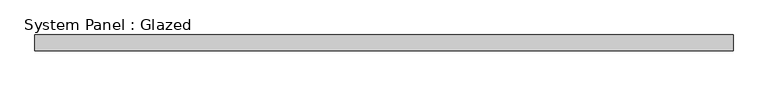
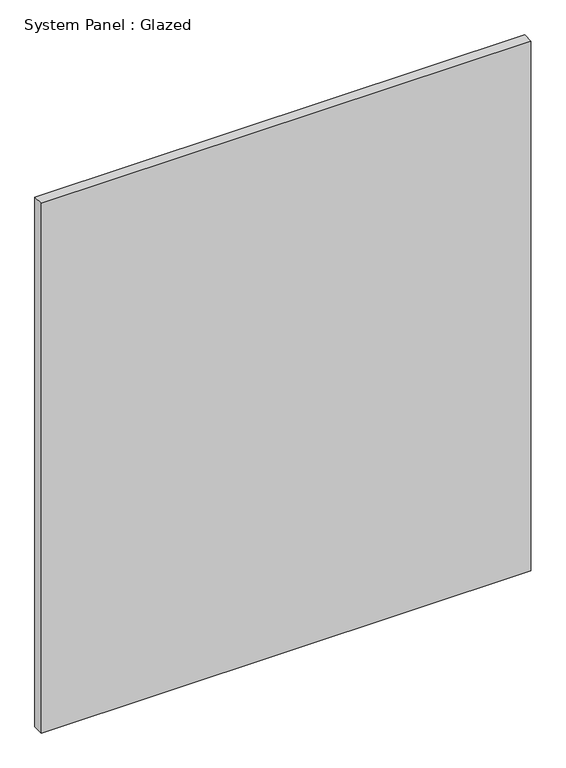
"""IFC4 building model written with IfcOpenShell, lengths in millimetres: plate geometry, System Panel : Glazed."""

from ifc_helpers import new_model, si_unit, origin, origin_with_axes, place, context, project, spatial, polyline, outline, extrude, source, transform, mapped, element, save


def system_panel_glazed_fcf423c9(model_context):
    return source(origin(), model_context, "Body", "SweptSolid", [
        extrude(outline(polyline([(565.1500001, 19.05), (-565.1500001, 19.05), (-565.1500001, 44.45), (565.1500001, 44.45), (565.1500001, 19.05)])), origin_with_axes(), (0.0, 0.0, 1.0), 1292.6724956),
    ])


if __name__ == "__main__":
    model = new_model("IFC4")
    model_context = context("Model", 3, world=origin())
    ifc_project = project(units=[si_unit("LENGTHUNIT", "METRE", prefix="MILLI")], contexts=[model_context])
    site = spatial("IfcSite", under=ifc_project)
    building = spatial("IfcBuilding", under=site)
    placement = place(None, origin())
    system_panel_glazed_shape = system_panel_glazed_fcf423c9(model_context)
    element("IfcPlate", 1, ObjectType="System Panel : Glazed", at=placement, inside=building, context=model_context, shape_type="MappedRepresentation", body=[
        mapped(system_panel_glazed_shape, transform((0.0, 0.0, 0.0), x_axis=(1.0, 0.0, 0.0), y_axis=(0.0, 1.0, 0.0), z_axis=(0.0, 0.0, 1.0))),
    ])
    save(model, "model.ifc")

# Revit data of these elements
# Type "System Panel : Glazed"
#   Construction Type Id = "GSP4R"
#   Analytic Construction = "1/8 in Pilkington single glazing"
#   Visual Light Transmittance = 0.9
#   Solar Heat Gain Coefficient = 0.86
#   Heat Transfer Coefficient (U) = 1.18115 BTU/(h·ft²·°F)
#   Define Thermal Properties by = 1
# Element 1 (IfcPlate, "System Panel : Glazed")
#   Materials on its faces: "Glass"
# Materials
#   "Glass": class "Glass", colour RGB 0 128 192, transparency 0.75, Description = "Soda Lime Glass", Cost = 0
